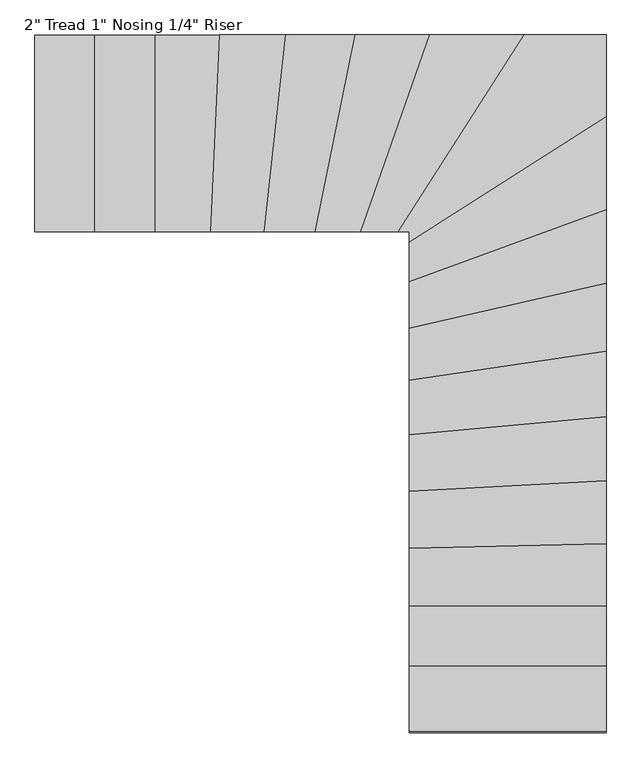
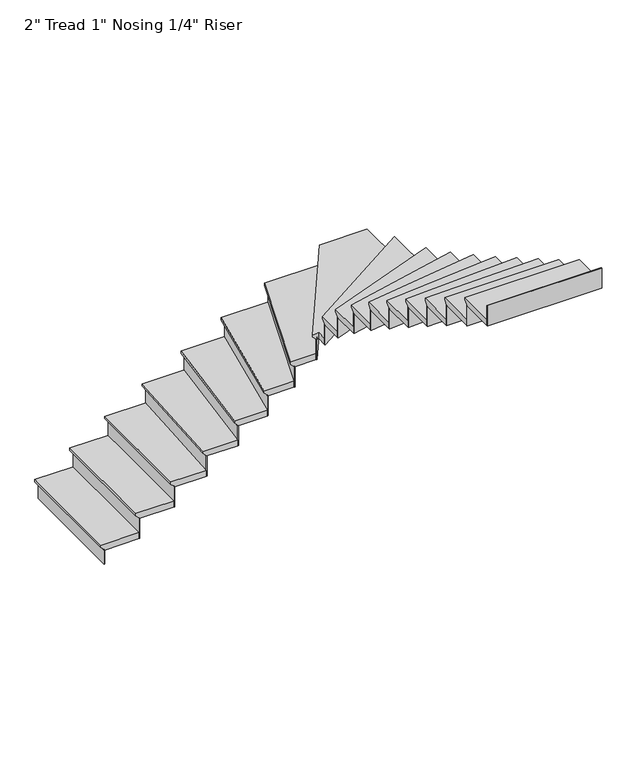
"""IFC4 building model written with IfcOpenShell, lengths in millimetres: stair flight geometry."""

from ifc_helpers import new_model, si_unit, origin, place, context, project, spatial, faceted_brep, source, transform, mapped, element, save


def stair_flight_bb54b32b(model_context):
    return source(origin(), model_context, "Body", "Brep", [
        faceted_brep([(-6926.0770189, 9644.7523405, 319.6166667), (-6926.0770189, 9644.7523405, 338.6666667), (-6926.0770189, 10559.1523405, 338.6666667), (-6926.0770189, 10559.1523405, 319.6166667), (-6900.6770189, 9644.7523405, 294.2166667), (-6900.6770189, 10559.1523405, 294.2166667), (-6621.2770189, 9644.7523405, 338.6666667), (-6621.2770189, 10559.1523405, 338.6666667), (-6900.6770189, 10559.1523405, 287.8666667), (-6621.2770189, 10559.1523405, 287.8666667), (-6621.2770189, 9644.7523405, 287.8666667), (-6900.6770189, 9644.7523405, 287.8666667)], [[[0, 1, 2, 3]], [[4, 0, 3, 5]], [[2, 1, 6, 7]], [[8, 9, 10, 11]], [[2, 7, 9, 8, 5, 3]], [[8, 11, 4, 5]], [[6, 1, 0, 4, 11, 10]], [[7, 6, 10, 9]]]),
        faceted_brep([(-6900.6770189, 9644.7523405, 287.8666667), (-6900.6770189, 9644.7523405, 169.3333333), (-6894.3270189, 9644.7523405, 169.3333333), (-6894.3270189, 9644.7523405, 287.8666667), (-6900.6770189, 10559.1523405, 287.8666667), (-6894.3270189, 10559.1523405, 287.8666667), (-6894.3270189, 10559.1523405, 169.3333333), (-6900.6770189, 10559.1523405, 169.3333333)], [[[0, 1, 2, 3]], [[4, 5, 6, 7]], [[1, 0, 4, 7]], [[2, 1, 7, 6]], [[3, 2, 6, 5]], [[0, 3, 5, 4]]]),
        faceted_brep([(-6621.2770189, 9644.7523405, 457.2), (-6621.2770189, 9644.7523405, 287.8666667), (-6614.9270189, 9644.7523405, 287.8666667), (-6614.9270189, 9644.7523405, 457.2), (-6621.2770189, 10559.1523405, 457.2), (-6614.9270189, 10559.1523405, 457.2), (-6614.9270189, 10559.1523405, 287.8666667), (-6621.2770189, 10559.1523405, 287.8666667)], [[[0, 1, 2, 3]], [[4, 5, 6, 7]], [[1, 0, 4, 7]], [[2, 1, 7, 6]], [[3, 2, 6, 5]], [[0, 3, 5, 4]]]),
        faceted_brep([(-6646.6770189, 10559.1523405, 508.0), (-6646.6770189, 9644.7523405, 508.0), (-6341.8770189, 9644.7523405, 508.0), (-6341.8770189, 10559.1523405, 508.0), (-6621.2770189, 10559.1523405, 457.2), (-6341.8770189, 10559.1523405, 457.2), (-6341.8770189, 9644.7523405, 457.2), (-6621.2770189, 9644.7523405, 457.2), (-6621.2770189, 10559.1523405, 463.55), (-6646.6770189, 10559.1523405, 488.95), (-6621.2770189, 9644.7523405, 463.55), (-6646.6770189, 9644.7523405, 488.95)], [[[0, 1, 2, 3]], [[4, 5, 6, 7]], [[0, 3, 5, 4, 8, 9]], [[4, 7, 10, 8]], [[2, 1, 11, 10, 7, 6]], [[3, 2, 6, 5]], [[11, 1, 0, 9]], [[10, 11, 9, 8]]]),
        faceted_brep([(-6341.8770189, 9644.7523405, 626.5333333), (-6341.8770189, 9644.7523405, 457.2), (-6335.5270189, 9644.7523405, 457.2), (-6335.5270189, 9644.7523405, 626.5333333), (-6341.8770189, 10559.1523405, 626.5333333), (-6335.5270189, 10559.1523405, 626.5333333), (-6335.5270189, 10559.1523405, 457.2), (-6341.8770189, 10559.1523405, 457.2)], [[[0, 1, 2, 3]], [[4, 5, 6, 7]], [[1, 0, 4, 7]], [[2, 1, 7, 6]], [[3, 2, 6, 5]], [[0, 3, 5, 4]]]),
        faceted_brep([(-6367.2770189, 10559.1523405, 677.3333333), (-6367.2770189, 9644.7523405, 677.3333333), (-6083.4472492, 9644.7523405, 677.3333333), (-6041.4532451, 10559.1523405, 677.3333333), (-6341.8770189, 10559.1523405, 626.5333333), (-6041.4532451, 10559.1523405, 626.5333333), (-6083.4472492, 9644.7523405, 626.5333333), (-6341.8770189, 9644.7523405, 626.5333333), (-6341.8770189, 10559.1523405, 632.8833333), (-6367.2770189, 10559.1523405, 658.2833333), (-6341.8770189, 9644.7523405, 632.8833333), (-6367.2770189, 9644.7523405, 658.2833333)], [[[0, 1, 2, 3]], [[4, 5, 6, 7]], [[0, 3, 5, 4, 8, 9]], [[4, 7, 10, 8]], [[2, 1, 11, 10, 7, 6]], [[3, 2, 6, 5]], [[11, 1, 0, 9]], [[10, 11, 9, 8]]]),
        faceted_brep([(-6083.4472492, 9644.7523405, 795.8666667), (-6083.4472492, 9644.7523405, 626.5333333), (-6077.0905563, 9644.7523405, 626.5333333), (-6077.0905563, 9644.7523405, 795.8666667), (-6041.4532451, 10559.1523405, 795.8666667), (-6035.0965522, 10559.1523405, 795.8666667), (-6035.0965522, 10559.1523405, 626.5333333), (-6041.4532451, 10559.1523405, 626.5333333)], [[[0, 1, 2, 3]], [[4, 5, 6, 7]], [[1, 0, 4, 7]], [[2, 1, 7, 6]], [[3, 2, 6, 5]], [[0, 3, 5, 4]]]),
        faceted_brep([(-6066.8800169, 10559.1523405, 846.6666667), (-6108.874021, 9644.7523405, 846.6666667), (-5832.8255301, 9644.7523405, 846.6666667), (-5733.0268439, 10559.1523405, 846.6666667), (-6041.4532451, 10559.1523405, 795.8666667), (-5733.0268439, 10559.1523405, 795.8666667), (-5832.8255301, 9644.7523405, 795.8666667), (-6083.4472492, 9644.7523405, 795.8666667), (-6041.4532451, 10559.1523405, 802.2166667), (-6066.8800169, 10559.1523405, 827.6166667), (-6083.4472492, 9644.7523405, 802.2166667), (-6108.874021, 9644.7523405, 827.6166667)], [[[0, 1, 2, 3]], [[4, 5, 6, 7]], [[0, 3, 5, 4, 8, 9]], [[4, 7, 10, 8]], [[2, 1, 11, 10, 7, 6]], [[3, 2, 6, 5]], [[11, 1, 0, 9]], [[10, 11, 9, 8]]]),
        faceted_brep([(-5832.8255301, 9644.7523405, 965.2), (-5832.8255301, 9644.7523405, 795.8666667), (-5826.4378221, 9644.7523405, 795.8666667), (-5826.4378221, 9644.7523405, 965.2), (-5733.0268439, 10559.1523405, 965.2), (-5726.6391359, 10559.1523405, 965.2), (-5726.6391359, 10559.1523405, 795.8666667), (-5733.0268439, 10559.1523405, 795.8666667)], [[[0, 1, 2, 3]], [[4, 5, 6, 7]], [[1, 0, 4, 7]], [[2, 1, 7, 6]], [[3, 2, 6, 5]], [[0, 3, 5, 4]]]),
        faceted_brep([(-5758.5776759, 10559.1523405, 1016.0), (-5858.376362, 9644.7523405, 1016.0), (-5595.3725014, 9644.7523405, 1016.0), (-5410.9587198, 10559.1523405, 1016.0), (-5733.0268439, 10559.1523405, 965.2), (-5410.9587198, 10559.1523405, 965.2), (-5595.3725014, 9644.7523405, 965.2), (-5832.8255301, 9644.7523405, 965.2), (-5733.0268439, 10559.1523405, 971.55), (-5758.5776759, 10559.1523405, 996.95), (-5832.8255301, 9644.7523405, 971.55), (-5858.376362, 9644.7523405, 996.95)], [[[0, 1, 2, 3]], [[4, 5, 6, 7]], [[0, 3, 5, 4, 8, 9]], [[4, 7, 10, 8]], [[2, 1, 11, 10, 7, 6]], [[3, 2, 6, 5]], [[11, 1, 0, 9]], [[10, 11, 9, 8]]]),
        faceted_brep([(-5595.3725014, 9644.7523405, 1134.5333333), (-5595.3725014, 9644.7523405, 965.2), (-5588.8946493, 9644.7523405, 965.2), (-5588.8946493, 9644.7523405, 1134.5333333), (-5410.9587198, 10559.1523405, 1134.5333333), (-5404.4808677, 10559.1523405, 1134.5333333), (-5404.4808677, 10559.1523405, 965.2), (-5410.9587198, 10559.1523405, 965.2)], [[[0, 1, 2, 3]], [[4, 5, 6, 7]], [[1, 0, 4, 7]], [[2, 1, 7, 6]], [[3, 2, 6, 5]], [[0, 3, 5, 4]]]),
        faceted_brep([(-5436.8701281, 10559.1523405, 1185.3333333), (-5621.2839097, 9644.7523405, 1185.3333333), (-5382.8270882, 9644.7523405, 1185.3333333), (-5062.7037856, 10559.1523405, 1185.3333333), (-5410.9587198, 10559.1523405, 1134.5333333), (-5062.7037856, 10559.1523405, 1134.5333333), (-5382.8270882, 9644.7523405, 1134.5333333), (-5595.3725014, 9644.7523405, 1134.5333333), (-5410.9587198, 10559.1523405, 1140.8833333), (-5436.8701281, 10559.1523405, 1166.2833333), (-5595.3725014, 9644.7523405, 1140.8833333), (-5621.2839097, 9644.7523405, 1166.2833333)], [[[0, 1, 2, 3]], [[4, 5, 6, 7]], [[0, 3, 5, 4, 8, 9]], [[4, 7, 10, 8]], [[2, 1, 11, 10, 7, 6]], [[3, 2, 6, 5]], [[11, 1, 0, 9]], [[10, 11, 9, 8]]]),
        faceted_brep([(-5382.8270882, 9644.7523405, 1303.8666667), (-5382.8270882, 9644.7523405, 1134.5333333), (-5376.0991927, 9644.7523405, 1134.5333333), (-5376.0991927, 9644.7523405, 1303.8666667), (-5062.7037856, 10559.1523405, 1303.8666667), (-5055.9758901, 10559.1523405, 1303.8666667), (-5055.9758901, 10559.1523405, 1134.5333333), (-5062.7037856, 10559.1523405, 1134.5333333)], [[[0, 1, 2, 3]], [[4, 5, 6, 7]], [[1, 0, 4, 7]], [[2, 1, 7, 6]], [[3, 2, 6, 5]], [[0, 3, 5, 4]]]),
        faceted_brep([(-5089.6153677, 10559.1523405, 1354.6666667), (-5409.7386702, 9644.7523405, 1354.6666667), (-5204.704396, 9644.7523405, 1354.6666667), (-4620.1049606, 10559.1523405, 1354.6666667), (-5062.7037856, 10559.1523405, 1303.8666667), (-4620.1049606, 10559.1523405, 1303.8666667), (-5204.704396, 9644.7523405, 1303.8666667), (-5382.8270882, 9644.7523405, 1303.8666667), (-5062.7037856, 10559.1523405, 1310.2166667), (-5089.6153677, 10559.1523405, 1335.6166667), (-5382.8270882, 9644.7523405, 1310.2166667), (-5409.7386702, 9644.7523405, 1335.6166667)], [[[0, 1, 2, 3]], [[4, 5, 6, 7]], [[0, 3, 5, 4, 8, 9]], [[4, 7, 10, 8]], [[2, 1, 11, 10, 7, 6]], [[3, 2, 6, 5]], [[11, 1, 0, 9]], [[10, 11, 9, 8]]]),
        faceted_brep([(-5204.704396, 9644.7523405, 1473.2), (-5204.704396, 9644.7523405, 1303.8666667), (-5197.1675656, 9644.7523405, 1303.8666667), (-5197.1675656, 9644.7523405, 1473.2), (-4620.1049606, 10559.1523405, 1473.2), (-4612.5681302, 10559.1523405, 1473.2), (-4612.5681302, 10559.1523405, 1303.8666667), (-4620.1049606, 10559.1523405, 1303.8666667)], [[[0, 1, 2, 3]], [[4, 5, 6, 7]], [[1, 0, 4, 7]], [[2, 1, 7, 6]], [[3, 2, 6, 5]], [[0, 3, 5, 4]]]),
        faceted_brep([(-4269.5400294, 10148.292766, 1524.0), (-4269.5400294, 10559.1523405, 1524.0), (-4650.2522823, 10559.1523405, 1524.0), (-5234.8517177, 9644.7523405, 1524.0), (-5183.9400294, 9644.7523405, 1524.0), (-5183.9400294, 9563.6933306, 1524.0), (-4269.5400294, 10559.1523405, 1473.2), (-4269.5400294, 10148.292766, 1473.2), (-5183.9400294, 9563.6933306, 1473.2), (-5183.9400294, 9644.7523405, 1473.2), (-5204.704396, 9644.7523405, 1473.2), (-4620.1049606, 10559.1523405, 1473.2), (-5204.704396, 9644.7523405, 1479.55), (-4620.1049606, 10559.1523405, 1479.55), (-5234.8517177, 9644.7523405, 1504.95), (-4650.2522823, 10559.1523405, 1504.95)], [[[0, 1, 2, 3, 4, 5]], [[6, 7, 8, 9, 10, 11]], [[1, 0, 7, 6]], [[11, 10, 12, 13]], [[4, 3, 14, 12, 10, 9]], [[0, 5, 8, 7]], [[14, 3, 2, 15]], [[12, 14, 15, 13]], [[2, 1, 6, 11, 13, 15]], [[5, 4, 9, 8]]]),
        faceted_brep([(-5183.9400294, 9563.6933306, 1642.5333333), (-5183.9400294, 9563.6933306, 1473.2), (-5183.9400294, 9556.1565002, 1473.2), (-5183.9400294, 9556.1565002, 1642.5333333), (-4269.5400294, 10148.292766, 1642.5333333), (-4269.5400294, 10140.7559356, 1642.5333333), (-4269.5400294, 10140.7559356, 1473.2), (-4269.5400294, 10148.292766, 1473.2)], [[[0, 1, 2, 3]], [[4, 5, 6, 7]], [[1, 0, 4, 7]], [[2, 1, 7, 6]], [[3, 2, 6, 5]], [[0, 3, 5, 4]]]),
        faceted_brep([(-4269.5400294, 10178.4400877, 1693.3333333), (-5183.9400294, 9593.8406523, 1693.3333333), (-5183.9400294, 9384.7373074, 1693.3333333), (-4269.5400294, 9719.2017424, 1693.3333333), (-4269.5400294, 10148.292766, 1642.5333333), (-4269.5400294, 9719.2017424, 1642.5333333), (-5183.9400294, 9384.7373074, 1642.5333333), (-5183.9400294, 9563.6933306, 1642.5333333), (-4269.5400294, 10148.292766, 1648.8833333), (-4269.5400294, 10178.4400877, 1674.2833333), (-5183.9400294, 9563.6933306, 1648.8833333), (-5183.9400294, 9593.8406523, 1674.2833333)], [[[0, 1, 2, 3]], [[4, 5, 6, 7]], [[0, 3, 5, 4, 8, 9]], [[4, 7, 10, 8]], [[2, 1, 11, 10, 7, 6]], [[3, 2, 6, 5]], [[11, 1, 0, 9]], [[10, 11, 9, 8]]]),
        faceted_brep([(-5183.9400294, 9384.7373074, 1811.8666667), (-5183.9400294, 9384.7373074, 1642.5333333), (-5183.9400294, 9377.9758508, 1642.5333333), (-5183.9400294, 9377.9758508, 1811.8666667), (-4269.5400294, 9719.2017424, 1811.8666667), (-4269.5400294, 9712.4402858, 1811.8666667), (-4269.5400294, 9712.4402858, 1642.5333333), (-4269.5400294, 9719.2017424, 1642.5333333)], [[[0, 1, 2, 3]], [[4, 5, 6, 7]], [[1, 0, 4, 7]], [[2, 1, 7, 6]], [[3, 2, 6, 5]], [[0, 3, 5, 4]]]),
        faceted_brep([(-4269.5400294, 9746.2475685, 1862.6666667), (-5183.9400294, 9411.7831335, 1862.6666667), (-5183.9400294, 9168.2180951, 1862.6666667), (-4269.5400294, 9378.8818777, 1862.6666667), (-4269.5400294, 9719.2017424, 1811.8666667), (-4269.5400294, 9378.8818777, 1811.8666667), (-5183.9400294, 9168.2180951, 1811.8666667), (-5183.9400294, 9384.7373074, 1811.8666667), (-4269.5400294, 9719.2017424, 1818.2166667), (-4269.5400294, 9746.2475685, 1843.6166667), (-5183.9400294, 9384.7373074, 1818.2166667), (-5183.9400294, 9411.7831335, 1843.6166667)], [[[0, 1, 2, 3]], [[4, 5, 6, 7]], [[0, 3, 5, 4, 8, 9]], [[4, 7, 10, 8]], [[2, 1, 11, 10, 7, 6]], [[3, 2, 6, 5]], [[11, 1, 0, 9]], [[10, 11, 9, 8]]]),
        faceted_brep([(-5183.9400294, 9168.2180951, 1981.2), (-5183.9400294, 9168.2180951, 1811.8666667), (-5183.9400294, 9161.7017539, 1811.8666667), (-5183.9400294, 9161.7017539, 1981.2), (-4269.5400294, 9378.8818777, 1981.2), (-4269.5400294, 9372.3655366, 1981.2), (-4269.5400294, 9372.3655366, 1811.8666667), (-4269.5400294, 9378.8818777, 1811.8666667)], [[[0, 1, 2, 3]], [[4, 5, 6, 7]], [[1, 0, 4, 7]], [[2, 1, 7, 6]], [[3, 2, 6, 5]], [[0, 3, 5, 4]]]),
        faceted_brep([(-4269.5400294, 9404.9472423, 2032.0), (-5183.9400294, 9194.2834597, 2032.0), (-5183.9400294, 8926.810153, 2032.0), (-4269.5400294, 9062.2661853, 2032.0), (-4269.5400294, 9378.8818777, 1981.2), (-4269.5400294, 9062.2661853, 1981.2), (-5183.9400294, 8926.810153, 1981.2), (-5183.9400294, 9168.2180951, 1981.2), (-4269.5400294, 9378.8818777, 1987.55), (-4269.5400294, 9404.9472423, 2012.95), (-5183.9400294, 9168.2180951, 1987.55), (-5183.9400294, 9194.2834597, 2012.95)], [[[0, 1, 2, 3]], [[4, 5, 6, 7]], [[0, 3, 5, 4, 8, 9]], [[4, 7, 10, 8]], [[2, 1, 11, 10, 7, 6]], [[3, 2, 6, 5]], [[11, 1, 0, 9]], [[10, 11, 9, 8]]]),
        faceted_brep([(-5183.9400294, 8926.810153, 2150.5333333), (-5183.9400294, 8926.810153, 1981.2), (-5183.9400294, 8920.3908576, 1981.2), (-5183.9400294, 8920.3908576, 2150.5333333), (-4269.5400294, 9062.2661853, 2150.5333333), (-4269.5400294, 9055.8468898, 2150.5333333), (-4269.5400294, 9055.8468898, 1981.2), (-4269.5400294, 9062.2661853, 1981.2)], [[[0, 1, 2, 3]], [[4, 5, 6, 7]], [[1, 0, 4, 7]], [[2, 1, 7, 6]], [[3, 2, 6, 5]], [[0, 3, 5, 4]]]),
        faceted_brep([(-4269.5400294, 9087.9433671, 2201.3333333), (-5183.9400294, 8952.4873349, 2201.3333333), (-5183.9400294, 8672.8434968, 2201.3333333), (-4269.5400294, 8757.7685803, 2201.3333333), (-4269.5400294, 9062.2661853, 2150.5333333), (-4269.5400294, 8757.7685803, 2150.5333333), (-5183.9400294, 8672.8434968, 2150.5333333), (-5183.9400294, 8926.810153, 2150.5333333), (-4269.5400294, 9062.2661853, 2156.8833333), (-4269.5400294, 9087.9433671, 2182.2833333), (-5183.9400294, 8926.810153, 2156.8833333), (-5183.9400294, 8952.4873349, 2182.2833333)], [[[0, 1, 2, 3]], [[4, 5, 6, 7]], [[0, 3, 5, 4, 8, 9]], [[4, 7, 10, 8]], [[2, 1, 11, 10, 7, 6]], [[3, 2, 6, 5]], [[11, 1, 0, 9]], [[10, 11, 9, 8]]]),
        faceted_brep([(-5183.9400294, 8672.8434968, 2319.8666667), (-5183.9400294, 8672.8434968, 2150.5333333), (-5183.9400294, 8666.4661687, 2150.5333333), (-5183.9400294, 8666.4661687, 2319.8666667), (-4269.5400294, 8757.7685803, 2319.8666667), (-4269.5400294, 8751.3912522, 2319.8666667), (-4269.5400294, 8751.3912522, 2150.5333333), (-4269.5400294, 8757.7685803, 2150.5333333)], [[[0, 1, 2, 3]], [[4, 5, 6, 7]], [[1, 0, 4, 7]], [[2, 1, 7, 6]], [[3, 2, 6, 5]], [[0, 3, 5, 4]]]),
        faceted_brep([(-4269.5400294, 8783.2778928, 2370.6666667), (-5183.9400294, 8698.3528093, 2370.6666667), (-5183.9400294, 8411.6607501, 2370.6666667), (-4269.5400294, 8460.2981403, 2370.6666667), (-4269.5400294, 8757.7685803, 2319.8666667), (-4269.5400294, 8460.2981403, 2319.8666667), (-5183.9400294, 8411.6607501, 2319.8666667), (-5183.9400294, 8672.8434968, 2319.8666667), (-4269.5400294, 8757.7685803, 2326.2166667), (-4269.5400294, 8783.2778928, 2351.6166667), (-5183.9400294, 8672.8434968, 2326.2166667), (-5183.9400294, 8698.3528093, 2351.6166667)], [[[0, 1, 2, 3]], [[4, 5, 6, 7]], [[0, 3, 5, 4, 8, 9]], [[4, 7, 10, 8]], [[2, 1, 11, 10, 7, 6]], [[3, 2, 6, 5]], [[11, 1, 0, 9]], [[10, 11, 9, 8]]]),
        faceted_brep([(-5183.9400294, 8411.6607501, 2489.2), (-5183.9400294, 8411.6607501, 2319.8666667), (-5183.9400294, 8405.3017736, 2319.8666667), (-5183.9400294, 8405.3017736, 2489.2), (-4269.5400294, 8460.2981403, 2489.2), (-4269.5400294, 8453.9391639, 2489.2), (-4269.5400294, 8453.9391639, 2319.8666667), (-4269.5400294, 8460.2981403, 2319.8666667)], [[[0, 1, 2, 3]], [[4, 5, 6, 7]], [[1, 0, 4, 7]], [[2, 1, 7, 6]], [[3, 2, 6, 5]], [[0, 3, 5, 4]]]),
        faceted_brep([(-4269.5400294, 8485.7340461, 2540.0), (-5183.9400294, 8437.0966559, 2540.0), (-5183.9400294, 8145.9511068, 2540.0), (-4269.5400294, 8167.2657958, 2540.0), (-4269.5400294, 8460.2981403, 2489.2), (-4269.5400294, 8167.2657958, 2489.2), (-5183.9400294, 8145.9511068, 2489.2), (-5183.9400294, 8411.6607501, 2489.2), (-4269.5400294, 8460.2981403, 2495.55), (-4269.5400294, 8485.7340461, 2520.95), (-5183.9400294, 8411.6607501, 2495.55), (-5183.9400294, 8437.0966559, 2520.95)], [[[0, 1, 2, 3]], [[4, 5, 6, 7]], [[0, 3, 5, 4, 8, 9]], [[4, 7, 10, 8]], [[2, 1, 11, 10, 7, 6]], [[3, 2, 6, 5]], [[11, 1, 0, 9]], [[10, 11, 9, 8]]]),
        faceted_brep([(-5183.9400294, 8145.9511068, 2658.5333333), (-5183.9400294, 8145.9511068, 2489.2), (-5183.9400294, 8139.5993819, 2489.2), (-5183.9400294, 8139.5993819, 2658.5333333), (-4269.5400294, 8167.2657958, 2658.5333333), (-4269.5400294, 8160.9140709, 2658.5333333), (-4269.5400294, 8160.9140709, 2489.2), (-4269.5400294, 8167.2657958, 2489.2)], [[[0, 1, 2, 3]], [[4, 5, 6, 7]], [[1, 0, 4, 7]], [[2, 1, 7, 6]], [[3, 2, 6, 5]], [[0, 3, 5, 4]]]),
        faceted_brep([(-4269.5400294, 8192.6726955, 2709.3333333), (-5183.9400294, 8171.3580065, 2709.3333333), (-5183.9400294, 7877.215351, 2709.3333333), (-4269.5400294, 7877.215351, 2709.3333333), (-4269.5400294, 8167.2657958, 2658.5333333), (-4269.5400294, 7877.215351, 2658.5333333), (-5183.9400294, 7877.215351, 2658.5333333), (-5183.9400294, 8145.9511068, 2658.5333333), (-4269.5400294, 8167.2657958, 2664.8833333), (-4269.5400294, 8192.6726955, 2690.2833333), (-5183.9400294, 8145.9511068, 2664.8833333), (-5183.9400294, 8171.3580065, 2690.2833333)], [[[0, 1, 2, 3]], [[4, 5, 6, 7]], [[0, 3, 5, 4, 8, 9]], [[4, 7, 10, 8]], [[2, 1, 11, 10, 7, 6]], [[3, 2, 6, 5]], [[11, 1, 0, 9]], [[10, 11, 9, 8]]]),
        faceted_brep([(-5183.9400294, 7877.215351, 2827.8666667), (-5183.9400294, 7877.215351, 2658.5333333), (-5183.9400294, 7870.865351, 2658.5333333), (-5183.9400294, 7870.865351, 2827.8666667), (-4269.5400294, 7877.215351, 2827.8666667), (-4269.5400294, 7870.865351, 2827.8666667), (-4269.5400294, 7870.865351, 2658.5333333), (-4269.5400294, 7877.215351, 2658.5333333)], [[[0, 1, 2, 3]], [[4, 5, 6, 7]], [[1, 0, 4, 7]], [[2, 1, 7, 6]], [[3, 2, 6, 5]], [[0, 3, 5, 4]]]),
        faceted_brep([(-4269.5400294, 7902.615351, 2878.6666667), (-5183.9400294, 7902.615351, 2878.6666667), (-5183.9400294, 7597.815351, 2878.6666667), (-4269.5400294, 7597.815351, 2878.6666667), (-4269.5400294, 7877.215351, 2827.8666667), (-4269.5400294, 7597.815351, 2827.8666667), (-5183.9400294, 7597.815351, 2827.8666667), (-5183.9400294, 7877.215351, 2827.8666667), (-4269.5400294, 7877.215351, 2834.2166667), (-4269.5400294, 7902.615351, 2859.6166667), (-5183.9400294, 7877.215351, 2834.2166667), (-5183.9400294, 7902.615351, 2859.6166667)], [[[0, 1, 2, 3]], [[4, 5, 6, 7]], [[0, 3, 5, 4, 8, 9]], [[4, 7, 10, 8]], [[2, 1, 11, 10, 7, 6]], [[3, 2, 6, 5]], [[11, 1, 0, 9]], [[10, 11, 9, 8]]]),
        faceted_brep([(-5183.9400294, 7597.815351, 2997.2), (-5183.9400294, 7597.815351, 2827.8666667), (-5183.9400294, 7591.465351, 2827.8666667), (-5183.9400294, 7591.465351, 2997.2), (-4269.5400294, 7597.815351, 2997.2), (-4269.5400294, 7591.465351, 2997.2), (-4269.5400294, 7591.465351, 2827.8666667), (-4269.5400294, 7597.815351, 2827.8666667)], [[[0, 1, 2, 3]], [[4, 5, 6, 7]], [[1, 0, 4, 7]], [[2, 1, 7, 6]], [[3, 2, 6, 5]], [[0, 3, 5, 4]]]),
        faceted_brep([(-5183.9400294, 7318.415351, 3166.5333333), (-5183.9400294, 7318.415351, 2997.2), (-5183.9400294, 7312.065351, 2997.2), (-5183.9400294, 7312.065351, 3166.5333333), (-4269.5400294, 7318.415351, 3166.5333333), (-4269.5400294, 7312.065351, 3166.5333333), (-4269.5400294, 7312.065351, 2997.2), (-4269.5400294, 7318.415351, 2997.2)], [[[0, 1, 2, 3]], [[4, 5, 6, 7]], [[1, 0, 4, 7]], [[2, 1, 7, 6]], [[3, 2, 6, 5]], [[0, 3, 5, 4]]]),
        faceted_brep([(-4269.5400294, 7623.215351, 3048.0), (-5183.9400294, 7623.215351, 3048.0), (-5183.9400294, 7318.415351, 3048.0), (-4269.5400294, 7318.415351, 3048.0), (-4269.5400294, 7597.815351, 2997.2), (-4269.5400294, 7318.415351, 2997.2), (-5183.9400294, 7318.415351, 2997.2), (-5183.9400294, 7597.815351, 2997.2), (-4269.5400294, 7597.815351, 3003.55), (-4269.5400294, 7623.215351, 3028.95), (-5183.9400294, 7597.815351, 3003.55), (-5183.9400294, 7623.215351, 3028.95)], [[[0, 1, 2, 3]], [[4, 5, 6, 7]], [[0, 3, 5, 4, 8, 9]], [[4, 7, 10, 8]], [[2, 1, 11, 10, 7, 6]], [[3, 2, 6, 5]], [[11, 1, 0, 9]], [[10, 11, 9, 8]]]),
    ])


if __name__ == "__main__":
    model = new_model("IFC4")
    model_context = context("Model", 3, world=origin())
    ifc_project = project(units=[si_unit("LENGTHUNIT", "METRE", prefix="MILLI")], contexts=[model_context])
    site = spatial("IfcSite", under=ifc_project)
    building = spatial("IfcBuilding", under=site)
    placement = place(None, origin())
    stair_flight_shape = stair_flight_bb54b32b(model_context)
    element("IfcStairFlight", 1, ObjectType="2\" Tread 1\" Nosing 1/4\" Riser", at=placement, inside=building, context=model_context, shape_type="MappedRepresentation", body=[
        mapped(stair_flight_shape, transform((0.0, 0.0, 0.0), x_axis=(1.0, 0.0, 0.0), y_axis=(0.0, 1.0, 0.0), z_axis=(0.0, 0.0, 1.0))),
    ])
    save(model, "model.ifc")
